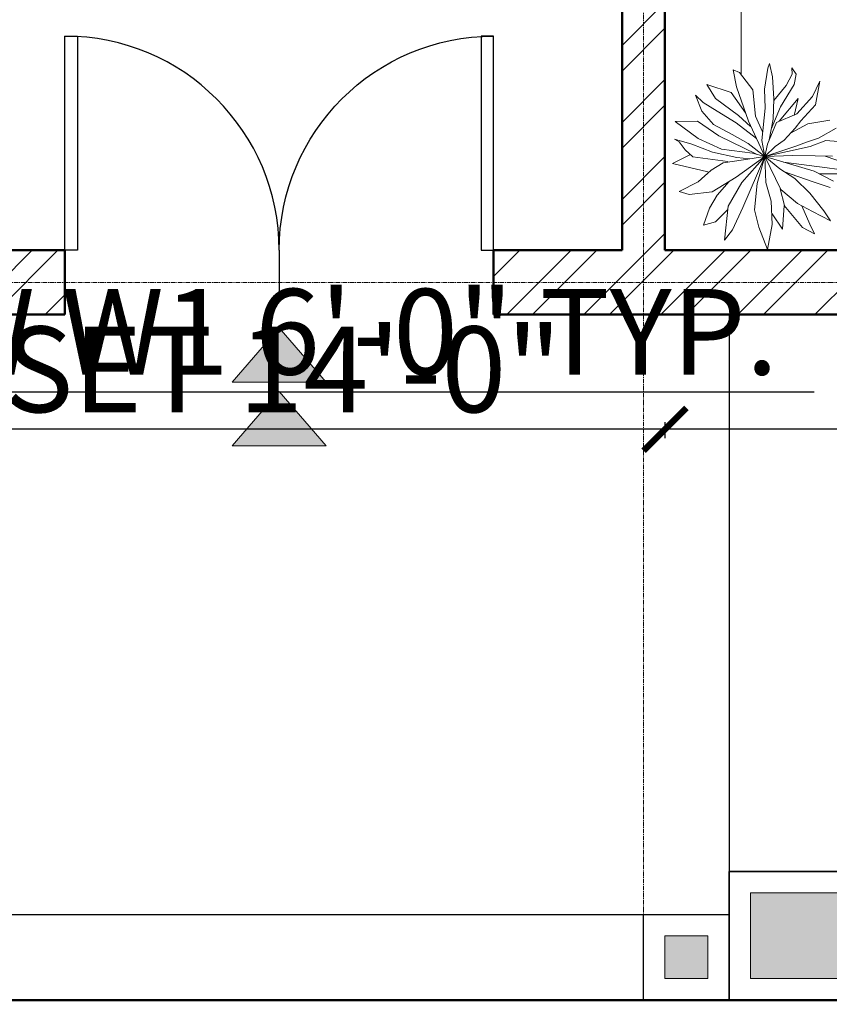
# Model space of a CAD drawing. Units: inches. Extents: x 261 to 2725, y 291 to 1454.
# Tile 8 of 35: x 688 to 801, y 412 to 550. Entities that reach past the tile are written whole.
import ezdxf

# ---------------------------------------------------------------- set-up
doc = ezdxf.new("R2010")
doc.units = ezdxf.units.IN
doc.linetypes.add('CENTER', pattern=[2, 1.25, -0.25, 0.25, -0.25])
for name, color, linetype, lineweight in [('A-ANNO-DIMS', 136, 'Continuous', 18), ('A-ANNO-SYMB', 7, 'Continuous', 18), ('A-DOOR', 160, 'Continuous', 25), ('A-FLOR-STRS', 42, 'Continuous', 25), ('A-FURN', 30, 'Continuous', 18), ('A-GRID', 251, 'CENTER', 13), ('A-PLNT', 3, 'Continuous', 18), ('A-PLNT-PATT', 3, 'Continuous', 13), ('A-WALL', 222, 'Continuous', 50), ('A-WALL-PATT', 243, 'Continuous', 13), ('C-PROP', 7, 'Continuous', 35)]:
    doc.layers.add(name, color=color, linetype=linetype, lineweight=lineweight)
doc.styles.get("Standard").update_dxf_attribs({"font": 'arial.ttf'})
doc.dimstyles.new('ISO-25', dxfattribs={"dimtxt": 12, "dimasz": 6, "dimexe": 1.25, "dimexo": 0.625, "dimtad": 1, "dimdec": 0, "dimlunit": 3, "dimtxsty": 'Standard', "dimblk": 'ARCHTICK', "dimcen": 2.5, "dimadec": 0, "dimazin": 0, "dimtfac": 1, "dimtdec": 0, "dimtmove": 0, "dimatfit": 3, "dimfxl": 1, "dimfxlon": 1, "dimarcsym": 0})

# ---------------------------------------------------------------- blocks, each defined once
blk = doc.blocks.new('*U11')
for p, q in [((0, 0), (0, -6)), ((30, 0), (30, -6))]:
    blk.add_line(p, q)
blk.add_lwpolyline([(0, 0), (0, 30), (1.75, 30), (1.75, 0)], close=True)
blk.add_arc((0, 0), 30, 0, 90)
blk = doc.blocks.new('A$C29956593')
for p, q in [((3602, 2800.7), (3586.8, 2719.3)), ((3630, 2728.1), (3602, 2800.7)), ((3447.8, 2749.3), (3463, 2718.1)), ((3486.3, 2729.3), (3447.8, 2749.3)), ((3742.2, 2770.6), (3716.5, 2736.8)), ((3730.5, 2659.2), (3742.2, 2770.6)), ((3463, 2718.1), (3488.7, 2658)), ((3547.1, 2656.7), (3486.3, 2729.3)), ((3551.8, 2734.3), (3547.1, 2656.7)), ((3586.8, 2684.2), (3551.8, 2734.3)), ((3586.8, 2719.3), (3589.1, 2643)), ((3644.1, 2670.5), (3630, 2728.1)), ((3716.5, 2736.8), (3682.6, 2663)), ((3811.1, 2721.8), (3772.6, 2710.5)), ((3792.4, 2665.5), (3811.1, 2721.8)), ((3395.2, 2706.8), (3416.2, 2674.3)), ((3453.6, 2676.8), (3395.2, 2706.8)), ((3772.6, 2710.5), (3732.8, 2670.5)), ((3416.2, 2674.3), (3463, 2616.7)), ((3502.7, 2650.5), (3453.6, 2676.8)), ((3557.6, 2604.2), (3502.7, 2650.5)), ((3545.9, 2656.7), (3559.9, 2601.7)), ((3682.6, 2663), (3610.3, 2495.9)), ((3635.9, 2584.1), (3644.1, 2670.5)), ((3686.1, 2581.6), (3730.5, 2659.2)), ((3766.7, 2622.9), (3792.4, 2665.5)), ((3589.1, 2643), (3606.7, 2581.6)), ((3727.7, 2578), (3766.7, 2622.9)), ((3859, 2620.4), (3783.1, 2611.7)), ((3891.7, 2610.4), (3859, 2620.4)), ((3454.8, 2577.9), (3396.4, 2597.9)), ((3463, 2616.7), (3512, 2567.8)), ((3610.3, 2495.9), (3557.6, 2604.2)), ((3783.1, 2611.7), (3704.8, 2564.1)), ((3828.6, 2579.1), (3891.7, 2610.4)), ((3384.7, 2576.6), (3448.9, 2544.1)), ((3545.4, 2546.5), (3454.8, 2577.9)), ((3512, 2567.8), (3561.1, 2536.6)), ((3606.7, 2581.6), (3610.3, 2495.9)), ((3610.3, 2495.9), (3635.9, 2584.1)), ((3610.3, 2495.9), (3686.1, 2581.6)), ((3704.8, 2564.1), (3610.3, 2495.9)), ((3786.6, 2540.3), (3828.6, 2579.1)), ((3431.3, 2553), (3240.6, 2553)), ((3342.6, 2541.6), (3405.7, 2532.8)), ((3405.7, 2532.8), (3548.9, 2514.2)), ((3448.9, 2544.1), (3610.3, 2495.9)), ((3561.1, 2536.6), (3610.3, 2495.9)), ((3746.9, 2516.5), (3786.6, 2540.3)), ((3912.8, 2519), (3797.1, 2546.6)), ((3412.7, 2494.7), (3339.1, 2520.3)), ((3388.2, 2495.2), (3445.4, 2494)), ((3445.4, 2494), (3517.9, 2492.7)), ((3610.3, 2495.9), (3461.8, 2462.7)), ((3508.5, 2461.5), (3610.3, 2495.9)), ((3517.9, 2492.7), (3610.3, 2495.9)), ((3576.3, 2462.7), (3610.3, 2495.9)), ((3610.3, 2495.9), (3602, 2455.2)), ((3610.3, 2495.9), (3680.3, 2506.5)), ((3610.3, 2495.9), (3651.1, 2485.2)), ((3663.9, 2380.1), (3610.3, 2495.9)), ((3610.3, 2495.9), (3620.7, 2443.9)), ((3665.1, 2452.7), (3610.3, 2495.9)), ((3702.5, 2499), (3660.1, 2503.8)), ((3680.3, 2506.5), (3746.9, 2516.5)), ((3781.9, 2481.5), (3702.5, 2499)), ((3731.7, 2512.8), (3846.2, 2496.5)), ((3846.2, 2496.5), (3871.9, 2474)), ((3853.9, 2489.7), (3912.8, 2519)), ((3461.8, 2462.7), (3410.4, 2443.9)), ((3473.5, 2448.9), (3508.5, 2461.5)), ((3547.1, 2442.7), (3576.3, 2462.7)), ((3760.9, 2427.6), (3637.7, 2488.7)), ((3651.1, 2485.2), (3752.7, 2471.5)), ((3752.7, 2471.5), (3828.6, 2436.4)), ((3849.7, 2455.2), (3781.9, 2481.5)), ((3871.9, 2474), (3891.7, 2447.7)), ((3410.4, 2443.9), (3369.5, 2446.4)), ((3376.5, 2402.6), (3433.8, 2435.2)), ((3433.8, 2435.2), (3473.5, 2448.9)), ((3510.9, 2402.6), (3547.1, 2442.7)), ((3602, 2455.2), (3571.6, 2383.8)), ((3583.3, 2373.8), (3596, 2441.2)), ((3620.7, 2443.9), (3609, 2337.5)), ((3637.7, 2436.6), (3704.8, 2385.1)), ((3717.7, 2423.9), (3665.1, 2452.7)), ((3831, 2380.1), (3760.9, 2427.6)), ((3828.6, 2436.4), (3904.6, 2381.3)), ((3906.9, 2438.9), (3849.7, 2455.2)), ((3891.7, 2447.7), (3906.9, 2438.9)), ((3526, 2419.4), (3468.8, 2388.9)), ((3492.2, 2378.8), (3510.9, 2402.6)), ((3558.8, 2332.5), (3589.6, 2405.9)), ((3617.5, 2415.2), (3640.5, 2363.8)), ((3696.6, 2361.3), (3656.9, 2397.6)), ((3778.4, 2391.4), (3717.7, 2423.9)), ((3468.8, 2388.9), (3397.5, 2376.3)), ((3444.3, 2326.3), (3492.2, 2378.8)), ((3563.4, 2380.1), (3500.4, 2305)), ((3500.4, 2305), (3514.4, 2361.3)), ((3571.6, 2383.8), (3505, 2356.3)), ((3581, 2306.2), (3583.3, 2373.8)), ((3640.5, 2363.8), (3649.9, 2277.4)), ((3703.6, 2267.4), (3663.9, 2380.1)), ((3772.6, 2305), (3696.6, 2361.3)), ((3704.8, 2385.1), (3766.7, 2347.5)), ((3816.9, 2347.5), (3778.4, 2391.4)), ((3904.6, 2381.3), (3831, 2380.1)), ((3505, 2356.3), (3453.6, 2298.7)), ((3514.4, 2259.9), (3558.8, 2332.5)), ((3609, 2337.5), (3611.3, 2274.9)), ((3673.6, 2352.7), (3721.2, 2286.2)), ((3766.7, 2347.5), (3812.3, 2318.8)), ((3838, 2295), (3816.9, 2347.5)), ((3430.2, 2248.7), (3444.3, 2326.3)), ((3453.6, 2298.7), (3430.2, 2248.7)), ((3581.2, 2312.4), (3540.1, 2262.4)), ((3585.6, 2234.9), (3581, 2306.2)), ((3800.6, 2259.9), (3772.6, 2305)), ((3812.3, 2318.8), (3838, 2295)), ((3611.3, 2274.9), (3600.8, 2206.1)), ((3649.9, 2277.4), (3693.1, 2219.9)), ((3714.1, 2211.1), (3703.6, 2267.4)), ((3721.2, 2286.2), (3800.6, 2259.9)), ((3507.4, 2226.1), (3514.4, 2259.9)), ((3540.1, 2262.4), (3520.2, 2226.1)), ((3595, 2191.1), (3585.6, 2234.9)), ((3521.4, 2204.8), (3507.4, 2226.1)), ((3520.2, 2226.1), (3521.4, 2204.8)), ((3600.8, 2206.1), (3595, 2191.1)), ((3687.6, 2019.2), (3687.6, 2227.2)), ((3693.1, 2219.9), (3714.1, 2211.1))]:
    blk.add_line(p, q)
blk = doc.blocks.new('_ArchTick')
at = {"color": 0, "linetype": 'ByBlock', "const_width": 0.15}
blk.add_lwpolyline([(-0.5, -0.5), (0.5, 0.5)], dxfattribs=at)
blk = doc.blocks.new('*D28')
at = {"layer": 'A-ANNO-DIMS', "color": 0, "lineweight": -2, "transparency": 16777216}
for p, q in [((469.45, 349.55), (469.45, 347.3)), ((955.45, 349.55), (955.45, 347.3)), ((469.45, 348.55), (955.45, 348.55))]:
    blk.add_line(p, q, dxfattribs=at)
at = {"layer": 'Defpoints', "color": 0, "transparency": 16777216}
for p in [(469.45, 508.47), (955.45, 508.47), (955.45, 348.55)]:
    blk.add_point(p, dxfattribs=at)
at = {"layer": 'A-ANNO-DIMS', "color": 0, "lineweight": -2, "transparency": 16777216, "xscale": 6, "yscale": 6, "zscale": 6, "rotation": 180}
blk.add_blockref('_ArchTick', (469.45, 348.55), dxfattribs=at)
at = {"layer": 'A-ANNO-DIMS', "color": 0, "lineweight": -2, "transparency": 16777216, "xscale": 6, "yscale": 6, "zscale": 6}
blk.add_blockref('_ArchTick', (955.45, 348.55), dxfattribs=at)
at = {"layer": 'A-ANNO-DIMS', "color": 0, "transparency": 16777216, "insert": (712.45, 355.3), "char_height": 12, "attachment_point": 5}
blk.add_mtext('40\'-6"', dxfattribs=at)
blk = doc.blocks.new('*D31')
at = {"layer": 'A-ANNO-DIMS', "color": 0, "lineweight": -2, "transparency": 16777216}
for p, q in [((478.45, 389.14), (478.45, 386.89)), ((946.45, 389.14), (946.45, 386.89)), ((478.45, 388.14), (946.45, 388.14))]:
    blk.add_line(p, q, dxfattribs=at)
at = {"layer": 'Defpoints', "color": 0, "transparency": 16777216}
for p in [(478.45, 517.47), (946.45, 517.47), (946.45, 388.14)]:
    blk.add_point(p, dxfattribs=at)
at = {"layer": 'A-ANNO-DIMS', "color": 0, "lineweight": -2, "transparency": 16777216, "xscale": 6, "yscale": 6, "zscale": 6, "rotation": 180}
blk.add_blockref('_ArchTick', (478.45, 388.14), dxfattribs=at)
at = {"layer": 'A-ANNO-DIMS', "color": 0, "lineweight": -2, "transparency": 16777216, "xscale": 6, "yscale": 6, "zscale": 6}
blk.add_blockref('_ArchTick', (946.45, 388.14), dxfattribs=at)
at = {"layer": 'A-ANNO-DIMS', "color": 0, "transparency": 16777216, "insert": (712.45, 394.89), "char_height": 12, "attachment_point": 5}
blk.add_mtext("39'", dxfattribs=at)
blk = doc.blocks.new('*D39')
at = {"layer": 'A-ANNO-DIMS', "color": 0, "lineweight": -2, "ltscale": 0.07, "transparency": 16777216}
for p, q in [((538.45, 498.67), (538.45, 496.42)), ((610.45, 498.67), (610.45, 496.42)), ((538.45, 497.67), (610.45, 497.67)), ((610.45, 497.67), (799.35, 497.67))]:
    blk.add_line(p, q, dxfattribs=at)
at = {"layer": 'Defpoints', "color": 0, "ltscale": 0.07, "transparency": 16777216}
for p in [(538.45, 508.47), (610.45, 508.47), (610.45, 497.67)]:
    blk.add_point(p, dxfattribs=at)
at = {"layer": 'A-ANNO-DIMS', "color": 0, "lineweight": -2, "ltscale": 0.07, "transparency": 16777216, "xscale": 6, "yscale": 6, "zscale": 6, "rotation": 180}
blk.add_blockref('_ArchTick', (538.45, 497.67), dxfattribs=at)
at = {"layer": 'A-ANNO-DIMS', "color": 0, "lineweight": -2, "ltscale": 0.07, "transparency": 16777216, "xscale": 6, "yscale": 6, "zscale": 6}
blk.add_blockref('_ArchTick', (610.45, 497.67), dxfattribs=at)
at = {"layer": 'A-ANNO-DIMS', "color": 0, "ltscale": 0.07, "transparency": 16777216, "insert": (707.9, 504.5), "char_height": 12, "attachment_point": 5}
blk.add_mtext('WINDOW W1 6\'-0" TYP.', dxfattribs=at)
blk = doc.blocks.new('*D67')
at = {"layer": 'A-ANNO-DIMS', "color": 0, "lineweight": -2, "ltscale": 0.07, "transparency": 16777216}
for p, q in [((778.45, 492.4), (526.52, 492.4)), ((778.45, 493.4), (778.45, 491.15)), ((946.45, 492.4), (778.45, 492.4)), ((946.45, 493.4), (946.45, 491.15))]:
    blk.add_line(p, q, dxfattribs=at)
at = {"layer": 'Defpoints', "color": 0, "ltscale": 0.07, "transparency": 16777216}
for p in [(778.45, 517.6), (946.45, 517.6), (778.45, 492.4)]:
    blk.add_point(p, dxfattribs=at)
at = {"layer": 'A-ANNO-DIMS', "color": 0, "lineweight": -2, "ltscale": 0.07, "transparency": 16777216, "xscale": 6, "yscale": 6, "zscale": 6, "rotation": 180}
blk.add_blockref('_ArchTick', (778.45, 492.4), dxfattribs=at)
at = {"layer": 'A-ANNO-DIMS', "color": 0, "lineweight": -2, "ltscale": 0.07, "transparency": 16777216, "xscale": 6, "yscale": 6, "zscale": 6}
blk.add_blockref('_ArchTick', (946.45, 492.4), dxfattribs=at)
at = {"layer": 'A-ANNO-DIMS', "color": 0, "ltscale": 0.07, "transparency": 16777216, "insert": (649.49, 499.24), "char_height": 12, "attachment_point": 5}
blk.add_mtext('LIVING ROOM SOFA SET 14\'-0"', dxfattribs=at)
blk = doc.blocks.new('*D86')
at = {"layer": 'A-ANNO-DIMS', "color": 0, "lineweight": -2, "ltscale": 0.07, "transparency": 16777216}
for p, q in [((676.45, 1437.76), (676.45, 1440.01)), ((772.45, 1437.76), (772.45, 1440.01)), ((676.45, 1438.76), (772.45, 1438.76))]:
    blk.add_line(p, q, dxfattribs=at)
at = {"layer": 'Defpoints', "color": 0, "ltscale": 0.07, "transparency": 16777216}
for p in [(772.45, 1438.76), (676.45, 517.47), (772.45, 517.47)]:
    blk.add_point(p, dxfattribs=at)
at = {"layer": 'A-ANNO-DIMS', "color": 0, "lineweight": -2, "ltscale": 0.07, "transparency": 16777216, "xscale": 6, "yscale": 6, "zscale": 6, "rotation": 180}
blk.add_blockref('_ArchTick', (676.45, 1438.76), dxfattribs=at)
at = {"layer": 'A-ANNO-DIMS', "color": 0, "lineweight": -2, "ltscale": 0.07, "transparency": 16777216, "xscale": 6, "yscale": 6, "zscale": 6}
blk.add_blockref('_ArchTick', (772.45, 1438.76), dxfattribs=at)
at = {"layer": 'A-ANNO-DIMS', "color": 0, "ltscale": 0.07, "transparency": 16777216, "insert": (724.45, 1445.51), "char_height": 12, "attachment_point": 5}
blk.add_mtext('8\'-0"', dxfattribs=at)
blk = doc.blocks.new('*D87')
at = {"layer": 'A-ANNO-DIMS', "color": 0, "lineweight": -2, "ltscale": 0.07, "transparency": 16777216}
for p, q in [((694.45, 305.22), (694.45, 302.97)), ((754.45, 305.22), (754.45, 302.97)), ((694.45, 304.22), (754.45, 304.22))]:
    blk.add_line(p, q, dxfattribs=at)
at = {"layer": 'Defpoints', "color": 0, "ltscale": 0.07, "transparency": 16777216}
for p in [(694.45, 508.47), (754.45, 508.47), (754.45, 304.22)]:
    blk.add_point(p, dxfattribs=at)
at = {"layer": 'A-ANNO-DIMS', "color": 0, "lineweight": -2, "ltscale": 0.07, "transparency": 16777216, "xscale": 6, "yscale": 6, "zscale": 6, "rotation": 180}
blk.add_blockref('_ArchTick', (694.45, 304.22), dxfattribs=at)
at = {"layer": 'A-ANNO-DIMS', "color": 0, "lineweight": -2, "ltscale": 0.07, "transparency": 16777216, "xscale": 6, "yscale": 6, "zscale": 6}
blk.add_blockref('_ArchTick', (754.45, 304.22), dxfattribs=at)
at = {"layer": 'A-ANNO-DIMS', "color": 0, "ltscale": 0.07, "transparency": 16777216, "insert": (724.45, 310.97), "char_height": 12, "attachment_point": 5}
blk.add_mtext('5\'-0"', dxfattribs=at)
blk = doc.blocks.new('*D88')
at = {"layer": 'A-ANNO-DIMS', "color": 0, "lineweight": -2, "ltscale": 0.07, "transparency": 16777216}
for p, q in [((430.45, 305.22), (430.45, 302.97)), ((994.45, 305.22), (994.45, 302.97)), ((430.45, 304.22), (994.45, 304.22))]:
    blk.add_line(p, q, dxfattribs=at)
at = {"layer": 'Defpoints', "color": 0, "ltscale": 0.07, "transparency": 16777216}
for p in [(430.45, 412.47), (994.45, 412.47), (994.45, 304.22)]:
    blk.add_point(p, dxfattribs=at)
at = {"layer": 'A-ANNO-DIMS', "color": 0, "lineweight": -2, "ltscale": 0.07, "transparency": 16777216, "xscale": 6, "yscale": 6, "zscale": 6, "rotation": 180}
blk.add_blockref('_ArchTick', (430.45, 304.22), dxfattribs=at)
at = {"layer": 'A-ANNO-DIMS', "color": 0, "lineweight": -2, "ltscale": 0.07, "transparency": 16777216, "xscale": 6, "yscale": 6, "zscale": 6}
blk.add_blockref('_ArchTick', (994.45, 304.22), dxfattribs=at)
at = {"layer": 'A-ANNO-DIMS', "color": 0, "ltscale": 0.07, "transparency": 16777216, "insert": (712.45, 310.97), "char_height": 12, "attachment_point": 5}
blk.add_mtext('47\'-0"', dxfattribs=at)
blk = doc.blocks.new('*D93')
at = {"layer": 'A-ANNO-DIMS', "color": 0, "lineweight": -2, "ltscale": 0.07, "transparency": 16777216}
for p, q in [((661.45, 305.22), (661.45, 302.97)), ((787.45, 305.22), (787.45, 302.97)), ((661.45, 304.22), (787.45, 304.22))]:
    blk.add_line(p, q, dxfattribs=at)
at = {"layer": 'Defpoints', "color": 0, "ltscale": 0.07, "transparency": 16777216}
for p in [(661.45, 430.47), (787.45, 430.47), (787.45, 304.22)]:
    blk.add_point(p, dxfattribs=at)
at = {"layer": 'A-ANNO-DIMS', "color": 0, "lineweight": -2, "ltscale": 0.07, "transparency": 16777216, "xscale": 6, "yscale": 6, "zscale": 6, "rotation": 180}
blk.add_blockref('_ArchTick', (661.45, 304.22), dxfattribs=at)
at = {"layer": 'A-ANNO-DIMS', "color": 0, "lineweight": -2, "ltscale": 0.07, "transparency": 16777216, "xscale": 6, "yscale": 6, "zscale": 6}
blk.add_blockref('_ArchTick', (787.45, 304.22), dxfattribs=at)
at = {"layer": 'A-ANNO-DIMS', "color": 0, "ltscale": 0.07, "transparency": 16777216, "insert": (724.45, 310.97), "char_height": 12, "attachment_point": 5}
blk.add_mtext('10\'-6"', dxfattribs=at)
blk = doc.blocks.new('*D103')
at = {"layer": 'A-ANNO-DIMS', "color": 0, "lineweight": -2, "ltscale": 0.07, "transparency": 16777216}
for p, q in [((287.06, 1231.47), (284.81, 1231.47)), ((286.06, 439.47), (286.06, 1231.47)), ((287.06, 439.47), (284.81, 439.47))]:
    blk.add_line(p, q, dxfattribs=at)
at = {"layer": 'Defpoints', "color": 0, "ltscale": 0.07, "transparency": 16777216}
for p in [(286.06, 1231.47), (1243.08, 1231.47), (1243.08, 439.47)]:
    blk.add_point(p, dxfattribs=at)
at = {"layer": 'A-ANNO-DIMS', "color": 0, "lineweight": -2, "ltscale": 0.07, "transparency": 16777216, "xscale": 6, "yscale": 6, "zscale": 6}
for p, rotation in [((286.06, 1231.47), 90), ((286.06, 439.47), 270)]:
    blk.add_blockref('_ArchTick', p, dxfattribs=dict(at, rotation=rotation))
at = {"layer": 'A-ANNO-DIMS', "color": 0, "ltscale": 0.07, "transparency": 16777216, "insert": (279.3, 835.47), "char_height": 12, "attachment_point": 5, "rotation": 90}
blk.add_mtext('66\'-0"', dxfattribs=at)
blk = doc.blocks.new('*D106')
at = {"layer": 'A-ANNO-DIMS', "color": 0, "lineweight": -2, "ltscale": 0.07, "transparency": 16777216}
for p, q in [((287.06, 496.47), (284.81, 496.47)), ((286.06, 448.47), (286.06, 496.47)), ((287.06, 448.47), (284.81, 448.47))]:
    blk.add_line(p, q, dxfattribs=at)
at = {"layer": 'Defpoints', "color": 0, "ltscale": 0.07, "transparency": 16777216}
for p in [(286.06, 496.47), (1252.08, 496.47), (1252.08, 448.47)]:
    blk.add_point(p, dxfattribs=at)
at = {"layer": 'A-ANNO-DIMS', "color": 0, "lineweight": -2, "ltscale": 0.07, "transparency": 16777216, "xscale": 6, "yscale": 6, "zscale": 6}
for p, rotation in [((286.06, 496.47), 90), ((286.06, 448.47), 270)]:
    blk.add_blockref('_ArchTick', p, dxfattribs=dict(at, rotation=rotation))
at = {"layer": 'A-ANNO-DIMS', "color": 0, "ltscale": 0.07, "transparency": 16777216, "insert": (279.3, 472.47), "char_height": 12, "attachment_point": 5, "rotation": 90}
blk.add_mtext('4\'-0"', dxfattribs=at)
blk = doc.blocks.new('*D107')
at = {"layer": 'A-ANNO-DIMS', "color": 0, "lineweight": -2, "ltscale": 0.07, "transparency": 16777216}
for p, q in [((287.06, 673.47), (284.81, 673.47)), ((286.06, 496.47), (286.06, 673.47)), ((287.06, 496.47), (284.81, 496.47))]:
    blk.add_line(p, q, dxfattribs=at)
at = {"layer": 'Defpoints', "color": 0, "ltscale": 0.07, "transparency": 16777216}
for p in [(286.06, 673.47), (1252.08, 673.47), (1252.08, 496.47)]:
    blk.add_point(p, dxfattribs=at)
at = {"layer": 'A-ANNO-DIMS', "color": 0, "lineweight": -2, "ltscale": 0.07, "transparency": 16777216, "xscale": 6, "yscale": 6, "zscale": 6}
for p, rotation in [((286.06, 673.47), 90), ((286.06, 496.47), 270)]:
    blk.add_blockref('_ArchTick', p, dxfattribs=dict(at, rotation=rotation))
at = {"layer": 'A-ANNO-DIMS', "color": 0, "ltscale": 0.07, "transparency": 16777216, "insert": (279.3, 584.97), "char_height": 12, "attachment_point": 5, "rotation": 90}
blk.add_mtext('14\'-9"', dxfattribs=at)
blk = doc.blocks.new('*D123')
at = {"layer": 'A-ANNO-DIMS', "color": 0, "lineweight": -2, "ltscale": 0.07, "transparency": 16777216}
for p, q in [((287.06, 1054.85), (284.81, 1054.85)), ((286.06, 439.47), (286.06, 1054.85)), ((287.06, 439.47), (284.81, 439.47))]:
    blk.add_line(p, q, dxfattribs=at)
at = {"layer": 'Defpoints', "color": 0, "ltscale": 0.07, "transparency": 16777216}
for p in [(286.06, 1054.85), (2007.71, 1054.85), (2007.71, 439.47)]:
    blk.add_point(p, dxfattribs=at)
at = {"layer": 'A-ANNO-DIMS', "color": 0, "lineweight": -2, "ltscale": 0.07, "transparency": 16777216, "xscale": 6, "yscale": 6, "zscale": 6}
for p, rotation in [((286.06, 1054.85), 90), ((286.06, 439.47), 270)]:
    blk.add_blockref('_ArchTick', p, dxfattribs=dict(at, rotation=rotation))
at = {"layer": 'A-ANNO-DIMS', "color": 0, "ltscale": 0.07, "transparency": 16777216, "insert": (279.22, 747.16), "char_height": 12, "attachment_point": 5, "rotation": 90}
blk.add_mtext('51\'-3 1/2"', dxfattribs=at)

msp = doc.modelspace()

# ---------------------------------------------------------------- hatches: boundary and pattern name
at = {"layer": 'A-ANNO-SYMB'}
h = msp.add_hatch(color=256, dxfattribs=at)
h.dxf.hatch_style = 1
h.paths.add_polyline_path([(1635.7, 825.23), (1627.39, 830.03), (1627.39, 820.43)])
h.paths.add_polyline_path([(1678.73, 860.77), (1673.94, 852.47), (1683.53, 852.47)])
h.paths.add_polyline_path([(1581.58, 805.28), (1576.78, 796.98), (1586.37, 796.98)])
h.paths.add_polyline_path([(724.45, 497.71), (717.86, 490.1), (731.04, 490.1)])
h.paths.add_polyline_path([(724.45, 506.59), (717.86, 498.98), (731.04, 498.98)])
at = {"layer": 'A-PLNT-PATT'}
h = msp.add_hatch(dxfattribs=at)
h.set_pattern_fill('GRASS', color=256, scale=0.7)
h.paths.add_polyline_path([(658.45, 427.47), (433.45, 427.47), (433.45, 415.47), (658.45, 415.47)])
h.paths.add_polyline_path([(670.45, 421.47), (664.45, 421.47), (664.45, 415.47), (670.45, 415.47)])
h.paths.add_polyline_path([(784.45, 421.47), (778.45, 421.47), (778.45, 415.47), (784.45, 415.47)])
h.paths.add_polyline_path([(991.45, 427.47), (790.45, 427.47), (790.45, 415.47), (991.45, 415.47)])
h.paths.add_polyline_path([(1439.08, 1220.47), (1252.08, 1220.47), (1252.08, 1198.47), (1417.08, 1198.47), (1417.08, 1117.47), (1439.08, 1117.47)])
h.paths.add_polyline_path([(2304.71, 1045.85), (2016.71, 1045.85), (2016.71, 805.87), (2304.71, 805.87)])
h.paths.add_polyline_path([(1267.21, 1201.68), (1431.59, 1201.68), (1431.59, 1218.76), (1267.21, 1218.76)], flags=24)
h.paths.add_polyline_path([(2089.2, 883.04), (2242.64, 883.04), (2242.64, 936.27), (2089.2, 936.27)], flags=24)
at = {"layer": 'A-WALL-PATT'}
h = msp.add_hatch(dxfattribs=at)
h.set_pattern_fill('ANSI32', color=256, scale=0.8)
h.paths.add_polyline_path([(478.45, 685.47), (580.45, 685.47), (580.45, 691.47), (577.45, 691.47), (577.45, 694.47), (571.45, 694.47), (571.45, 691.47), (478.45, 691.47), (478.45, 721.47), (469.45, 721.47), (469.45, 508.47), (538.45, 508.47), (538.45, 517.47), (478.45, 517.47)])
h.paths.add_polyline_path([(694.45, 517.47), (676.45, 517.47), (676.45, 646.47), (670.45, 646.47), (670.45, 517.47), (610.45, 517.47), (610.45, 508.47), (694.45, 508.47)])
h.paths.add_polyline_path([(676.45, 784.47), (478.45, 784.47), (478.45, 844.47), (469.45, 844.47), (469.45, 745.47), (478.45, 745.47), (478.45, 775.47), (571.45, 775.47), (571.45, 724.47), (577.45, 724.47), (577.45, 775.47), (670.45, 775.47), (670.45, 691.47), (610.45, 691.47), (610.45, 685.47), (670.45, 685.47), (670.45, 682.47), (676.45, 682.47)])
h.paths.add_polyline_path([(955.45, 880.47), (946.45, 880.47), (946.45, 808.47), (778.45, 808.47), (778.45, 799.47), (946.45, 799.47), (946.45, 517.47), (898.45, 517.47), (898.45, 508.47), (955.45, 508.47)])
h.paths.add_polyline_path([(778.45, 598.47), (772.45, 598.47), (772.45, 517.47), (754.45, 517.47), (754.45, 508.47), (826.45, 508.47), (826.45, 517.47), (778.45, 517.47)])
h.paths.add_polyline_path([(955.45, 1090.47), (946.45, 1090.47), (946.45, 1030.47), (817.45, 1030.47), (817.45, 1024.47), (946.45, 1024.47), (946.45, 952.47), (955.45, 952.47)])
h.paths.add_polyline_path([(955.45, 1231.47), (730.45, 1231.47), (730.45, 1222.47), (772.45, 1222.47), (772.45, 1096.47), (766.45, 1096.47), (766.45, 1090.47), (772.45, 1090.47), (772.45, 1006.47), (712.45, 1006.47), (712.45, 1000.47), (778.45, 1000.47), (778.45, 1024.47), (781.45, 1024.47), (781.45, 1030.47), (778.45, 1030.47), (778.45, 1222.47), (946.45, 1222.47), (946.45, 1162.47), (955.45, 1162.47)])
h.paths.add_polyline_path([(694.45, 1231.47), (619.45, 1231.47), (619.45, 1222.47), (646.45, 1222.47), (646.45, 1039.47), (652.45, 1039.47), (652.45, 1090.47), (736.45, 1090.47), (736.45, 1096.47), (652.45, 1096.47), (652.45, 1222.47), (694.45, 1222.47)])
h.paths.add_polyline_path([(571.45, 1231.47), (469.45, 1231.47), (469.45, 1099.47), (478.45, 1099.47), (478.45, 1144.47), (544.45, 1144.47), (544.45, 1153.47), (538.45, 1153.47), (538.45, 1150.47), (478.45, 1150.47), (478.45, 1222.47), (538.45, 1222.47), (538.45, 1183.47), (544.45, 1183.47), (544.45, 1222.47), (571.45, 1222.47)])
h.paths.add_polyline_path([(538.45, 1006.47), (478.45, 1006.47), (478.45, 1051.47), (469.45, 1051.47), (469.45, 940.47), (478.45, 940.47), (478.45, 1000.47), (538.45, 1000.47)])
h.paths.add_polyline_path([(652.45, 1006.47), (652.45, 1009.47), (646.45, 1009.47), (646.45, 1006.47), (586.45, 1006.47), (586.45, 1000.47), (652.45, 1000.47)])
h.paths.add_polyline_path([(1288.08, 973.47), (1243.08, 973.47), (1243.08, 920.97), (1252.08, 920.97), (1252.08, 964.47), (1288.08, 964.47)], flags=17)
h.paths.add_polyline_path([(1402.08, 805.47), (1252.08, 805.47), (1252.08, 848.97), (1243.08, 848.97), (1243.08, 757.47), (1252.08, 757.47), (1252.08, 799.47), (1294.08, 799.47), (1372.08, 799.47), (1372.08, 779.47), (1372.08, 715.47), (1378.08, 715.47), (1378.08, 799.47), (1402.08, 799.47)])
h.paths.add_polyline_path([(1252.08, 721.47), (1243.08, 721.47), (1243.08, 439.47), (1729.08, 439.47), (1729.08, 709.47), (1720.08, 709.47), (1720.08, 679.47), (1582.08, 679.47), (1582.08, 670.47), (1588.08, 670.47), (1588.08, 673.47), (1720.08, 673.47), (1720.08, 559.47), (1690.08, 559.47), (1690.08, 550.47), (1720.08, 550.47), (1720.08, 448.47), (1252.08, 448.47), (1252.08, 496.47), (1312.08, 496.47), (1312.08, 505.47), (1252.08, 505.47), (1252.08, 673.47), (1405.08, 673.47), (1405.08, 679.47), (1378.08, 679.47), (1378.08, 685.47), (1372.08, 685.47), (1372.08, 679.47), (1252.08, 679.47)])
h.paths.add_polyline_path([(1450.08, 550.47), (1480.08, 550.47), (1480.08, 559.47), (1450.08, 559.47), (1450.08, 679.47), (1441.08, 679.47), (1441.08, 673.47), (1444.08, 673.47), (1444.08, 505.47), (1384.08, 505.47), (1384.08, 496.47), (1450.08, 496.47)], flags=17)
h.paths.add_polyline_path([(1618.08, 559.47), (1588.08, 559.47), (1588.08, 634.47), (1582.08, 634.47), (1582.08, 559.47), (1552.08, 559.47), (1552.08, 550.47), (1618.08, 550.47)], flags=17)
h.paths.add_polyline_path([(1564.08, 964.47), (1630.08, 964.47), (1630.08, 973.47), (1477.08, 973.47), (1477.08, 964.47), (1558.08, 964.47), (1558.08, 926.22), (1558.08, 887.97), (1486.08, 887.97), (1486.08, 881.97), (1558.08, 881.97), (1558.08, 805.47), (1450.08, 805.47), (1450.08, 845.97), (1444.08, 845.97), (1444.08, 805.47), (1438.08, 805.47), (1438.08, 799.47), (1564.08, 799.47)], flags=17)
h.paths.add_polyline_path([(1453.08, 973.47), (1408.08, 973.47), (1408.08, 964.47), (1444.08, 964.47), (1444.08, 881.97), (1450.08, 881.97), (1456.08, 881.97), (1456.08, 887.97), (1450.08, 887.97), (1450.08, 964.47), (1453.08, 964.47)], flags=17)
h.paths.add_polyline_path([(1729.08, 1231.47), (1243.08, 1231.47), (1243.08, 1167.47), (1252.08, 1167.47), (1252.08, 1222.47), (1441.08, 1222.47), (1441.08, 1045.47), (1648.08, 1045.47), (1648.08, 1051.47), (1450.08, 1051.47), (1450.08, 1074.47), (1450.08, 1222.47), (1472.08, 1222.47), (1720.08, 1222.47), (1720.08, 1051.47), (1708.08, 1051.47), (1708.08, 1045.47), (1720.08, 1045.47), (1720.08, 973.47), (1702.08, 973.47), (1702.08, 964.47), (1720.08, 964.47), (1720.08, 769.47), (1729.08, 769.47)])
h.paths.add_polyline_path([(2493.71, 1054.85), (2007.71, 1054.85), (2007.71, 439.47), (2214.67, 439.47), (2214.67, 496.47), (2493.71, 496.47)])
h.paths.add_polyline_path([(2016.71, 1045.85), (2304.71, 1045.85), (2304.71, 841.47), (2310.71, 841.47), (2310.71, 1045.85), (2484.71, 1045.85), (2484.71, 805.47), (2310.71, 805.47), (2310.71, 811.47), (2304.71, 811.47), (2304.71, 799.47), (2484.71, 799.47), (2484.71, 679.47), (2304.71, 679.47), (2304.71, 673.47), (2484.71, 673.47), (2484.71, 505.47), (2208.67, 505.47), (2208.67, 448.47), (2016.71, 448.47), (2016.71, 799.47), (2304.71, 799.47), (2304.71, 805.47), (2016.71, 805.47)], flags=16)

# ---------------------------------------------------------------- linework, layer by layer
at = {"layer": 'A-ANNO-SYMB'}
for points in [[(731.04, 498.98), (724.45, 506.59), (717.86, 498.98)], [(731.04, 490.1), (724.45, 497.71), (717.86, 490.1)]]:
    msp.add_lwpolyline(points, close=True, dxfattribs=at)
at = {"layer": 'A-FLOR-STRS'}
for p, q in [((787.45, 508.47), (787.45, 412.47)), ((673.45, 424.47), (775.45, 424.47)), ((661.45, 412.47), (787.45, 412.47))]:
    msp.add_line(p, q, dxfattribs=at)
msp.add_lwpolyline([(787.45, 412.47), (775.45, 412.47), (775.45, 424.47), (787.45, 424.47)], close=True, dxfattribs=at)
at = {"layer": 'A-GRID', "ltscale": 0.5}
for p, q in [((775.45, 1330.47), (775.45, 416.47)), ((394.31, 512.97), (1018.31, 512.97))]:
    msp.add_line(p, q, dxfattribs=at)
at = {"layer": 'A-PLNT'}
for points in [[(790.45, 415.47), (991.45, 415.47), (991.45, 427.47), (790.45, 427.47)], [(784.45, 415.47), (778.45, 415.47), (778.45, 421.47), (784.45, 421.47)]]:
    msp.add_lwpolyline(points, close=True, dxfattribs=at)
at = {"layer": 'A-WALL'}
for p, q in [((772.45, 517.47), (772.45, 598.47)), ((778.45, 517.47), (778.45, 598.47)), ((676.45, 517.47), (694.45, 517.47)), ((694.45, 517.47), (694.45, 508.47)), ((754.45, 517.47), (754.45, 508.47)), ((754.45, 517.47), (772.45, 517.47)), ((778.45, 517.47), (826.45, 517.47)), ((610.45, 508.47), (694.45, 508.47)), ((754.45, 508.47), (826.45, 508.47)), ((430.45, 412.47), (994.45, 412.47))]:
    msp.add_line(p, q, dxfattribs=at)
at = {"layer": 'C-PROP'}
msp.add_lwpolyline([(787.45, 412.47), (994.45, 412.47), (994.45, 430.47), (787.45, 430.47)], close=True, dxfattribs=at)

# ---------------------------------------------------------------- block references
at = {"layer": 'A-DOOR'}
msp.add_blockref('*U11', (694.45, 517.47), dxfattribs=at)
at = {"layer": 'A-DOOR', "xscale": -1}
msp.add_blockref('*U11', (754.45, 517.47), dxfattribs=at)
at = {"layer": 'A-FURN', "xscale": 0.0426601237233356, "yscale": 0.0426601237233356, "zscale": 0.0426601237233356, "rotation": 180}
msp.add_blockref('A$C29956593', (946.45, 637.08), dxfattribs=at)

# ---------------------------------------------------------------- dimensions: what is measured, and where the dimension line sits
at = {"layer": 'A-ANNO-DIMS', "ltscale": 0.07}
for base, p1, p2, picture, middle in [((772.45, 1438.76), (676.45, 517.47), (772.45, 517.47), '*D86', (724.45, 1445.51)), ((754.45, 304.22), (694.45, 508.47), (754.45, 508.47), '*D87', (724.45, 310.97)), ((787.45, 304.22), (661.45, 430.47), (787.45, 430.47), '*D93', (724.45, 310.97)), ((994.45, 304.22), (430.45, 412.47), (994.45, 412.47), '*D88', (712.45, 310.97))]:
    dim = msp.add_linear_dim(base=base, p1=p1, p2=p2, dimstyle='ISO-25', override={"dimdec": 1, "dimlfac": 1, "dimrnd": 0, "dimzin": 1, "dimdsep": 46, "dimlunit": 4, "dimfrac": 2}, dxfattribs=at)
    dim.commit()
    dim.dimension.update_dxf_attribs({"geometry": picture, "text_midpoint": middle})
for base, p1, p2, picture, middle in [((286.06, 1231.47), (1243.08, 439.47), (1243.08, 1231.47), '*D103', (279.3, 835.47)), ((286.06, 1054.85), (2007.71, 439.47), (2007.71, 1054.85), '*D123', (279.22, 747.16)), ((286.06, 673.47), (1252.08, 496.47), (1252.08, 673.47), '*D107', (279.3, 584.97)), ((286.06, 496.47), (1252.08, 448.47), (1252.08, 496.47), '*D106', (279.3, 472.47))]:
    dim = msp.add_linear_dim(base=base, p1=p1, p2=p2, angle=90, dimstyle='ISO-25', override={"dimdec": 1, "dimlfac": 1, "dimrnd": 0, "dimzin": 1, "dimdsep": 46, "dimlunit": 4, "dimfrac": 2}, dxfattribs=at)
    dim.commit()
    dim.dimension.update_dxf_attribs({"geometry": picture, "text_midpoint": middle})
dim = msp.add_linear_dim(base=(778.45, 492.4), p1=(946.45, 517.6), p2=(778.45, 517.6), angle=180, text='LIVING ROOM SOFA SET <>', dimstyle='ISO-25', override={"dimdec": 1, "dimrnd": 0, "dimzin": 1, "dimlunit": 4, "dimfrac": 2}, dxfattribs=at)
dim.commit()
dim.dimension.update_dxf_attribs({"geometry": '*D67', "text_midpoint": (649.49, 499.24)})
dim = msp.add_linear_dim(base=(610.45, 497.67), p1=(538.45, 508.47), p2=(610.45, 508.47), text='WINDOW W1 <> TYP.', dimstyle='ISO-25', override={"dimdec": 1, "dimrnd": 0, "dimzin": 1, "dimlunit": 4, "dimfrac": 2}, dxfattribs=at)
dim.commit()
dim.dimension.update_dxf_attribs({"geometry": '*D39', "text_midpoint": (707.9, 504.5)})
at = {"layer": 'A-ANNO-DIMS'}
for base, p1, p2, picture, middle in [((946.45, 388.14), (478.45, 517.47), (946.45, 517.47), '*D31', (712.45, 388.14)), ((955.45, 348.55), (469.45, 508.47), (955.45, 508.47), '*D28', (712.45, 348.55))]:
    dim = msp.add_linear_dim(base=base, p1=p1, p2=p2, dimstyle='ISO-25', override={"dimclrd": 0, "dimclre": 0, "dimclrt": 0}, dxfattribs=at)
    dim.commit()
    dim.dimension.update_dxf_attribs({"geometry": picture, "text_midpoint": middle, "dimtype": 160})

doc.saveas('drawing.dxf')
